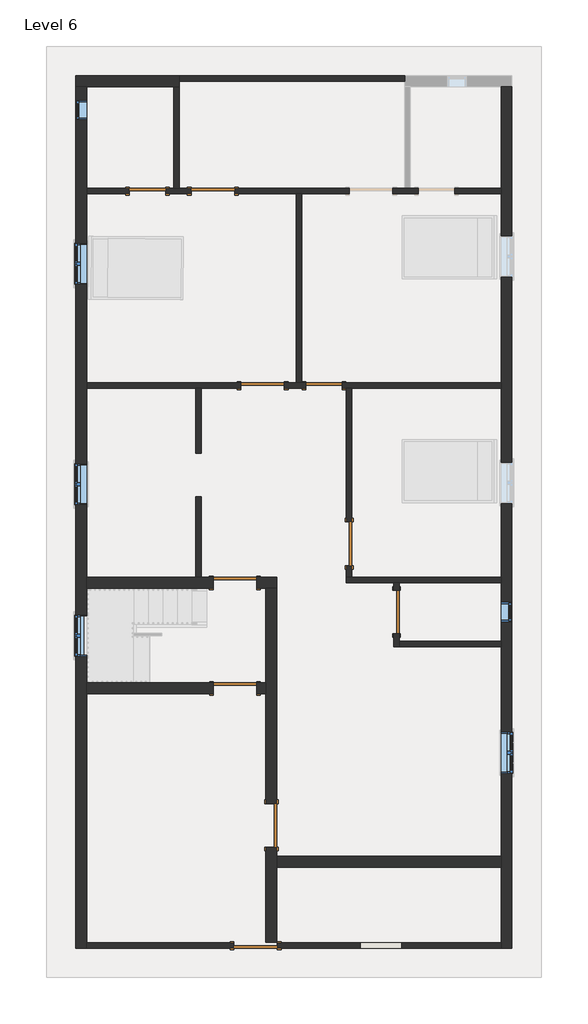
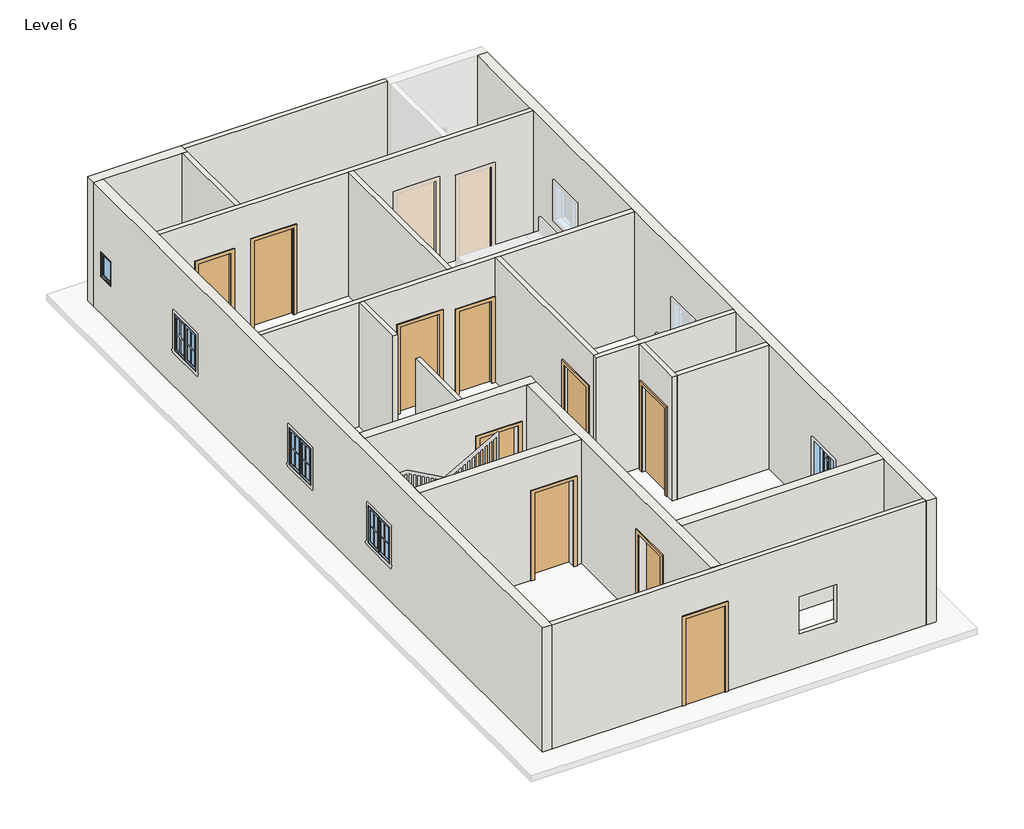
# One storey, part 1 of 3: 19 walls, 10 doors, 6 windows.
"""IFC4 building model written with IfcOpenShell, lengths in millimetres."""

from ifc_helpers import new_model, si_unit, frame, origin, place, context, project, spatial, polyline, outline, extrude, faceted_brep, transform, mapped, element, save
from components import door_d8f5dbb5, door_f2b275c1, door_e5f9f3c4, door_0ca8825f, door_305aa2a5, window_aa618e30, window_339605e1

model = new_model("IFC4")

# Units and contexts
model_context = context("Model", 3, world=origin())
ifc_project = project(units=[si_unit("LENGTHUNIT", "METRE", prefix="MILLI")], contexts=[model_context])

# Site, building, storey
site = spatial("IfcSite", under=ifc_project)
building = spatial("IfcBuilding", under=site)
storey = spatial("IfcBuildingStorey", under=building, Name="Level 6", Elevation=12801.6)

# Doors
placement = place(None, origin())
door_shape = door_d8f5dbb5(model_context)
element("IfcDoor", 1, ObjectType="Single-Flush : 30\" x 80\"", at=placement, inside=storey, context=model_context, shape_type="MappedRepresentation", body=[
    mapped(door_shape, transform((-4322.2915084, 8007.7072267, 12801.6), x_axis=(1.0, 0.0, 0.0), y_axis=(0.0, 1.0, 0.0), z_axis=(0.0, 0.0, 1.0))),
])
door_2_shape = door_f2b275c1(model_context)
element("IfcDoor", 2, ObjectType="Single-Flush : 30\" x 80\"", at=placement, inside=storey, context=model_context, shape_type="MappedRepresentation", body=[
    mapped(door_2_shape, transform((-621.124692, 3931.0072267, 12801.6), x_axis=(-1.0, 0.0, 0.0), y_axis=(0.0, -1.0, 0.0), z_axis=(0.0, 0.0, 1.0))),
])
door_3_shape = door_e5f9f3c4(model_context)
element("IfcDoor", 3, ObjectType="Single-Flush : 36\" x 84\"", at=placement, inside=storey, context=model_context, shape_type="MappedRepresentation", body=[
    mapped(door_3_shape, transform((-1909.2915084, 3931.0072267, 12801.6), x_axis=(1.0, 0.0, 0.0), y_axis=(0.0, 1.0, 0.0), z_axis=(0.0, 0.0, 1.0))),
])
element("IfcDoor", 4, ObjectType="Single-Flush : 36\" x 84\"", at=placement, inside=storey, context=model_context, shape_type="MappedRepresentation", body=[
    mapped(door_3_shape, transform((-94.9578757, 616.3072267, 12801.6), x_axis=(0.0, -1.0, 0.0), y_axis=(1.0, 0.0, 0.0), z_axis=(0.0, 0.0, 1.0))),
])
element("IfcDoor", 5, ObjectType="Single-Flush : 36\" x 84\"", at=placement, inside=storey, context=model_context, shape_type="MappedRepresentation", body=[
    mapped(door_3_shape, transform((-2055.3415084, -7803.7927733, 12801.6), x_axis=(-1.0, 0.0, 0.0), y_axis=(0.0, -1.0, 0.0), z_axis=(0.0, 0.0, 1.0))),
])
door_4_shape = door_0ca8825f(model_context)
element("IfcDoor", 6, ObjectType="Single-Flush : 36\" x 84\"", at=placement, inside=storey, context=model_context, shape_type="MappedRepresentation", body=[
    mapped(door_4_shape, transform((-2490.3165084, -202.8427733, 12801.6), x_axis=(1.0, 0.0, 0.0), y_axis=(0.0, 1.0, 0.0), z_axis=(0.0, 0.0, 1.0))),
])
element("IfcDoor", 7, ObjectType="Single-Flush : 36\" x 84\"", at=placement, inside=storey, context=model_context, shape_type="MappedRepresentation", body=[
    mapped(door_4_shape, transform((-2487.1415084, -2412.6427733, 12801.6), x_axis=(1.0, 0.0, 0.0), y_axis=(0.0, 1.0, 0.0), z_axis=(0.0, 0.0, 1.0))),
])
element("IfcDoor", 8, ObjectType="Single-Flush : 36\" x 84\"", at=placement, inside=storey, context=model_context, shape_type="MappedRepresentation", body=[
    mapped(door_4_shape, transform((-1725.1415084, -5282.8427733, 12801.6), x_axis=(0.0, -1.0, 0.0), y_axis=(1.0, 0.0, 0.0), z_axis=(0.0, 0.0, 1.0))),
])
door_5_shape = door_305aa2a5(model_context)
element("IfcDoor", 9, ObjectType="Single-Flush : 36\" x 84\"", at=placement, inside=storey, context=model_context, shape_type="MappedRepresentation", body=[
    mapped(door_5_shape, transform((897.4084916, -812.4427733, 12801.6), x_axis=(0.0, 1.0, 0.0), y_axis=(-1.0, 0.0, 0.0), z_axis=(0.0, 0.0, 1.0))),
])
element("IfcDoor", 10, ObjectType="Single-Flush : 36\" x 84\"", at=placement, inside=storey, context=model_context, shape_type="MappedRepresentation", body=[
    mapped(door_5_shape, transform((-2950.6915084, 8007.7072267, 12801.6), x_axis=(-1.0, 0.0, 0.0), y_axis=(0.0, -1.0, 0.0), z_axis=(0.0, 0.0, 1.0))),
])

# Walls
element("IfcWall", 11, ObjectType="WALL4.5\"", at=placement, inside=storey, context=model_context, shape_type="Brep", body=[
    faceted_brep([(821.2084916, 7950.5572267, 14935.2), (821.2084916, 7950.5572267, 12801.6), (1354.6084916, 7950.5572267, 12801.6), (1354.6084916, 7950.5572267, 14833.6), (2116.6084916, 7950.5572267, 14833.6), (2116.6084916, 7950.5572267, 12801.6), (3088.1584916, 7950.5572267, 12801.6), (3088.1584916, 7950.5572267, 15849.6), (-1090.1415084, 7950.5572267, 15849.6), (-1204.4415084, 7950.5572267, 15849.6), (-5598.6415084, 7950.5572267, 15849.6), (-5598.6415084, 7950.5572267, 12801.6), (-4703.2915084, 7950.5572267, 12801.6), (-4703.2915084, 7950.5572267, 14833.6), (-3941.2915084, 7950.5572267, 14833.6), (-3941.2915084, 7950.5572267, 12801.6), (-3407.8915084, 7950.5572267, 12801.6), (-3407.8915084, 7950.5572267, 14935.2), (-2493.4915084, 7950.5572267, 14935.2), (-2493.4915084, 7950.5572267, 12801.6), (-1204.4415084, 7950.5572267, 12801.6), (-1090.1415084, 7950.5572267, 12801.6), (-93.1915084, 7950.5572267, 12801.6), (-93.1915084, 7950.5572267, 14935.2), (1354.6084916, 8064.8572267, 12801.6), (1183.1584916, 8064.8572267, 12801.6), (1068.8584916, 8064.8572267, 12801.6), (821.2084916, 8064.8572267, 12801.6), (821.2084916, 8064.8572267, 14935.2), (-93.1915084, 8064.8572267, 14935.2), (-93.1915084, 8064.8572267, 12801.6), (-2493.4915084, 8064.8572267, 12801.6), (-2493.4915084, 8064.8572267, 14935.2), (-3407.8915084, 8064.8572267, 14935.2), (-3407.8915084, 8064.8572267, 12801.6), (-3655.5415084, 8064.8572267, 12801.6), (-3769.8415084, 8064.8572267, 12801.6), (-3941.2915084, 8064.8572267, 12801.6), (-3941.2915084, 8064.8572267, 14833.6), (-4703.2915084, 8064.8572267, 14833.6), (-4703.2915084, 8064.8572267, 12801.6), (-5598.6415084, 8064.8572267, 12801.6), (-5598.6415084, 8064.8572267, 15849.6), (-3769.8415084, 8064.8572267, 15849.6), (-3655.5415084, 8064.8572267, 15849.6), (1068.8584916, 8064.8572267, 15849.6), (1183.1584916, 8064.8572267, 15849.6), (3088.1584916, 8064.8572267, 15849.6), (3088.1584916, 8064.8572267, 12801.6), (2116.6084916, 8064.8572267, 12801.6), (2116.6084916, 8064.8572267, 14833.6), (1354.6084916, 8064.8572267, 14833.6)], [[[0, 1, 2, 3, 4, 5, 6, 7, 8, 9, 10, 11, 12, 13, 14, 15, 16, 17, 18, 19, 20, 21, 22, 23]], [[24, 25, 26, 27, 28, 29, 30, 31, 32, 33, 34, 35, 36, 37, 38, 39, 40, 41, 42, 43, 44, 45, 46, 47, 48, 49, 50, 51]], [[12, 11, 41, 40]], [[49, 48, 6, 5]], [[37, 36, 35, 34, 16, 15]], [[2, 1, 27, 26, 25, 24]], [[22, 21, 20, 19, 31, 30]], [[11, 10, 42, 41]], [[7, 6, 48, 47]], [[38, 37, 15, 14]], [[39, 38, 14, 13]], [[40, 39, 13, 12]], [[3, 2, 24, 51]], [[4, 3, 51, 50]], [[5, 4, 50, 49]], [[17, 16, 34, 33]], [[18, 17, 33, 32]], [[19, 18, 32, 31]], [[28, 27, 1, 0]], [[29, 28, 0, 23]], [[30, 29, 23, 22]], [[10, 9, 8, 7, 47, 46, 45, 44, 43, 42]]]),
])
element("IfcWall", 12, ObjectType="WALL4.5\"", at=placement, inside=storey, context=model_context, shape_type="SweptSolid", body=[
    extrude(outline(polyline([(-3769.8415084, 8064.8572267), (-3769.8415084, 10198.4572267), (-3655.5415084, 10198.4572267), (-3655.5415084, 8064.8572267), (-3769.8415084, 8064.8572267)])), frame((0.0, 0.0, 12801.6), z_axis=(0.0, 0.0, 1.0), x_axis=(1.0, 0.0, 0.0)), (0.0, 0.0, 1.0), 3048.0),
])
element("IfcWall", 13, ObjectType="WALL4.5\"", at=placement, inside=storey, context=model_context, shape_type="SweptSolid", body=[
    extrude(outline(polyline([(-1204.4415084, 3988.1572267), (-1204.4415084, 7950.5572267), (-1090.1415084, 7950.5572267), (-1090.1415084, 3988.1572267), (-1204.4415084, 3988.1572267)])), frame((0.0, 0.0, 12801.6), z_axis=(0.0, 0.0, 1.0), x_axis=(1.0, 0.0, 0.0)), (0.0, 0.0, 1.0), 3048.0),
])
element("IfcWall", 14, ObjectType="WALL4.5\"", at=placement, inside=storey, context=model_context, shape_type="Brep", body=[
    faceted_brep([(-1452.0915084, 3873.8572267, 12801.6), (-1002.124692, 3873.8572267, 12801.6), (-1002.124692, 3873.8572267, 14833.6), (-240.124692, 3873.8572267, 14833.6), (-240.124692, 3873.8572267, 12801.6), (-152.1078757, 3873.8572267, 12801.6), (-37.8078757, 3873.8572267, 12801.6), (3088.1584916, 3873.8572267, 12801.6), (3088.1584916, 3873.8572267, 15849.6), (-37.8078757, 3873.8572267, 15849.6), (-152.1078757, 3873.8572267, 15849.6), (-3198.3415084, 3873.8572267, 15849.6), (-3312.6415084, 3873.8572267, 15849.6), (-5598.6415084, 3873.8572267, 15849.6), (-5598.6415084, 3873.8572267, 12801.6), (-3312.6415084, 3873.8572267, 12801.6), (-3198.3415084, 3873.8572267, 12801.6), (-2366.4915084, 3873.8572267, 12801.6), (-2366.4915084, 3873.8572267, 14935.2), (-1452.0915084, 3873.8572267, 14935.2), (-1002.124692, 3988.1572267, 14833.6), (-1002.124692, 3988.1572267, 12801.6), (-1090.1415084, 3988.1572267, 12801.6), (-1204.4415084, 3988.1572267, 12801.6), (-1452.0915084, 3988.1572267, 12801.6), (-1452.0915084, 3988.1572267, 14935.2), (-2366.4915084, 3988.1572267, 14935.2), (-2366.4915084, 3988.1572267, 12801.6), (-5598.6415084, 3988.1572267, 12801.6), (-5598.6415084, 3988.1572267, 15849.6), (-1204.4415084, 3988.1572267, 15849.6), (-1090.1415084, 3988.1572267, 15849.6), (3088.1584916, 3988.1572267, 15849.6), (3088.1584916, 3988.1572267, 12801.6), (-240.124692, 3988.1572267, 12801.6), (-240.124692, 3988.1572267, 14833.6)], [[[0, 1, 2, 3, 4, 5, 6, 7, 8, 9, 10, 11, 12, 13, 14, 15, 16, 17, 18, 19]], [[20, 21, 22, 23, 24, 25, 26, 27, 28, 29, 30, 31, 32, 33, 34, 35]], [[17, 16, 15, 14, 28, 27]], [[34, 33, 7, 6, 5, 4]], [[24, 23, 22, 21, 1, 0]], [[14, 13, 29, 28]], [[8, 7, 33, 32]], [[25, 24, 0, 19]], [[26, 25, 19, 18]], [[27, 26, 18, 17]], [[2, 1, 21, 20]], [[3, 2, 20, 35]], [[4, 3, 35, 34]], [[13, 12, 11, 10, 9, 8, 32, 31, 30, 29]]]),
])
element("IfcWall", 15, ObjectType="WALL4.5\"", at=placement, inside=storey, context=model_context, shape_type="SweptSolid", body=[
    extrude(outline(polyline([(-3312.6415084, 2514.5843832), (-3312.6415084, 3873.8572267), (-3198.3415084, 3873.8572267), (-3198.3415084, 2514.5843832), (-3312.6415084, 2514.5843832)])), frame((0.0, 0.0, 12801.6), z_axis=(0.0, 0.0, 1.0), x_axis=(1.0, 0.0, 0.0)), (0.0, 0.0, 1.0), 3048.0),
])
element("IfcWall", 16, ObjectType="WALL4.5\"", at=placement, inside=storey, context=model_context, shape_type="SweptSolid", body=[
    extrude(outline(polyline([(-3312.6415084, -88.5427733), (-3312.6415084, 1600.2092553), (-3198.3415084, 1600.2092553), (-3198.3415084, -88.5427733), (-3312.6415084, -88.5427733)])), frame((0.0, 0.0, 12801.6), z_axis=(0.0, 0.0, 1.0), x_axis=(1.0, 0.0, 0.0)), (0.0, 0.0, 1.0), 3048.0),
])
element("IfcWall", 17, ObjectType="WALL4.5\"", at=placement, inside=storey, context=model_context, shape_type="SweptSolid", body=[
    extrude(outline(polyline([(159.1072267, 14935.2), (159.1072267, 12801.6), (-88.5427733, 12801.6), (-88.5427733, 15849.6), (3873.8572267, 15849.6), (3873.8572267, 12801.6), (1073.5072267, 12801.6), (1073.5072267, 14935.2), (159.1072267, 14935.2)])), frame((-152.1078757, 0.0, 0.0), z_axis=(1.0, 0.0, 0.0), x_axis=(0.0, 1.0, 0.0)), (0.0, 0.0, 1.0), 114.3),
])
element("IfcWall", 18, ObjectType="WALL4.5\"", at=placement, inside=storey, context=model_context, shape_type="Brep", body=[
    faceted_brep([(-152.1078757, -202.8427733, 12801.6), (840.2584916, -202.8427733, 12801.6), (954.5584916, -202.8427733, 12801.6), (3088.1584916, -202.8427733, 12801.6), (3088.1584916, -202.8427733, 15849.6), (954.5584916, -202.8427733, 15849.6), (840.2584916, -202.8427733, 15849.6), (-152.1078757, -202.8427733, 15849.6), (-152.1078757, -88.5427733, 12801.6), (-152.1078757, -88.5427733, 15849.6), (-37.8078757, -88.5427733, 15849.6), (3088.1584916, -88.5427733, 15849.6), (3088.1584916, -88.5427733, 12801.6), (-37.8078757, -88.5427733, 12801.6)], [[[0, 1, 2, 3, 4, 5, 6, 7]], [[8, 9, 10, 11, 12, 13]], [[3, 2, 1, 0, 8, 13, 12]], [[4, 3, 12, 11]], [[0, 7, 9, 8]], [[7, 6, 5, 4, 11, 10, 9]]]),
])
element("IfcWall", 19, ObjectType="WALL4.5\"", at=placement, inside=storey, context=model_context, shape_type="Brep", body=[
    faceted_brep([(840.2584916, -202.8427733, 12801.6), (840.2584916, -355.2427733, 12801.6), (840.2584916, -355.2427733, 14935.2), (840.2584916, -1269.6427733, 14935.2), (840.2584916, -1269.6427733, 12801.6), (840.2584916, -1536.3427733, 12801.6), (840.2584916, -1536.3427733, 15849.6), (840.2584916, -202.8427733, 15849.6), (954.5584916, -355.2427733, 14935.2), (954.5584916, -355.2427733, 12801.6), (954.5584916, -202.8427733, 12801.6), (954.5584916, -202.8427733, 15849.6), (954.5584916, -1422.0427733, 15849.6), (954.5584916, -1536.3427733, 15849.6), (954.5584916, -1536.3427733, 12801.6), (954.5584916, -1422.0427733, 12801.6), (954.5584916, -1269.6427733, 12801.6), (954.5584916, -1269.6427733, 14935.2)], [[[0, 1, 2, 3, 4, 5, 6, 7]], [[8, 9, 10, 11, 12, 13, 14, 15, 16, 17]], [[10, 9, 1, 0]], [[16, 15, 14, 5, 4]], [[0, 7, 11, 10]], [[6, 5, 14, 13]], [[2, 1, 9, 8]], [[3, 2, 8, 17]], [[4, 3, 17, 16]], [[7, 6, 13, 12, 11]]]),
])
element("IfcWall", 20, ObjectType="WALL4.5\"", at=placement, inside=storey, context=model_context, shape_type="SweptSolid", body=[
    extrude(outline(polyline([(3088.1584916, -1536.3427733), (954.5584916, -1536.3427733), (954.5584916, -1422.0427733), (3088.1584916, -1422.0427733), (3088.1584916, -1536.3427733)])), frame((0.0, 0.0, 12801.6), z_axis=(0.0, 0.0, 1.0), x_axis=(1.0, 0.0, 0.0)), (0.0, 0.0, 1.0), 3048.0),
])
element("IfcWall", 21, ObjectType="WALL4.5\"", at=placement, inside=storey, context=model_context, shape_type="SweptSolid", body=[
    extrude(outline(polyline([(12801.6, -5598.6415084), (12801.6, -2512.5415084), (14935.2, -2512.5415084), (14935.2, -1598.1415084), (12801.6, -1598.1415084), (12801.6, 3088.1584916), (15849.6, 3088.1584916), (15849.6, -5598.6415084), (12801.6, -5598.6415084)]), holes=[polyline([(14526.3479476, 141.7584916), (14526.3479476, 1005.3584916), (13611.9479476, 1005.3584916), (13611.9479476, 141.7584916), (14526.3479476, 141.7584916)])]), frame((0.0, -7860.9427733, 0.0), z_axis=(0.0, 1.0, 0.0), x_axis=(0.0, 0.0, 1.0)), (0.0, 0.0, 1.0), 114.3),
])
element("IfcWall", 22, ObjectType="WALL4.5\"", at=placement, inside=storey, context=model_context, shape_type="SweptSolid", body=[
    extrude(outline(polyline([(1068.8584916, 10312.7572267), (-3655.5415084, 10312.7572267), (-3655.5415084, 10427.0572267), (1068.8584916, 10427.0572267), (1068.8584916, 10312.7572267)])), frame((0.0, 0.0, 12801.6), z_axis=(0.0, 0.0, 1.0), x_axis=(1.0, 0.0, 0.0)), (0.0, 0.0, 1.0), 3048.0),
])
element("IfcWall", 23, ObjectType="WALL9\"", at=placement, inside=storey, context=model_context, shape_type="Brep", body=[
    faceted_brep([(-3655.5415084, 10427.0572267, 12801.6), (-5827.2415084, 10427.0572267, 12801.6), (-5827.2415084, 10427.0572267, 15849.6), (-3655.5415084, 10427.0572267, 15849.6), (-3655.5415084, 10198.4572267, 12801.6), (-3655.5415084, 10198.4572267, 15849.6), (-3769.8415084, 10198.4572267, 15849.6), (-5598.6415084, 10198.4572267, 15849.6), (-5827.2415084, 10198.4572267, 15849.6), (-5827.2415084, 10198.4572267, 12801.6), (-5598.6415084, 10198.4572267, 12801.6), (-3769.8415084, 10198.4572267, 12801.6), (-3655.5415084, 10312.7572267, 12801.6), (-3655.5415084, 10312.7572267, 15849.6)], [[[0, 1, 2, 3]], [[4, 5, 6, 7, 8, 9, 10, 11]], [[1, 0, 12, 4, 11, 10, 9]], [[2, 1, 9, 8]], [[0, 3, 13, 5, 4, 12]], [[3, 2, 8, 7, 6, 5, 13]]]),
])
element("IfcWall", 24, ObjectType="WALL9\"", at=placement, inside=storey, context=model_context, shape_type="Brep", body=[
    faceted_brep([(-5827.2415084, 10198.4572267, 12801.6), (-5827.2415084, -7860.9427733, 12801.6), (-5827.2415084, -7860.9427733, 15849.6), (-5827.2415084, 10198.4572267, 15849.6), (-5827.2415084, 9906.3572267, 14325.6), (-5827.2415084, 9499.9572267, 14325.6), (-5827.2415084, 9499.9572267, 13716.0), (-5827.2415084, 9906.3572267, 13716.0), (-5827.2415084, 6915.5072267, 14630.4), (-5827.2415084, 6051.9072267, 14630.4), (-5827.2415084, 6051.9072267, 13716.0), (-5827.2415084, 6915.5072267, 13716.0), (-5827.2415084, 2295.8822267, 14630.4), (-5827.2415084, 1432.2822267, 14630.4), (-5827.2415084, 1432.2822267, 13716.0), (-5827.2415084, 2295.8822267, 13716.0), (-5827.2415084, -875.9427733, 14630.4), (-5827.2415084, -1739.5427733, 14630.4), (-5827.2415084, -1739.5427733, 13716.0), (-5827.2415084, -875.9427733, 13716.0), (-5598.6415084, 10198.4572267, 12801.6), (-5598.6415084, 10198.4572267, 15849.6), (-5598.6415084, 8064.8572267, 15849.6), (-5598.6415084, 7950.5572267, 15849.6), (-5598.6415084, 3988.1572267, 15849.6), (-5598.6415084, 3873.8572267, 15849.6), (-5598.6415084, -88.5427733, 15849.6), (-5598.6415084, -317.1427733, 15849.6), (-5598.6415084, -2298.3427733, 15849.6), (-5598.6415084, -2526.9427733, 15849.6), (-5598.6415084, -7746.6427733, 15849.6), (-5598.6415084, -7860.9427733, 15849.6), (-5598.6415084, -7860.9427733, 12801.6), (-5598.6415084, -7746.6427733, 12801.6), (-5598.6415084, -2526.9427733, 12801.6), (-5598.6415084, -2298.3427733, 12801.6), (-5598.6415084, -317.1427733, 12801.6), (-5598.6415084, -88.5427733, 12801.6), (-5598.6415084, 3873.8572267, 12801.6), (-5598.6415084, 3988.1572267, 12801.6), (-5598.6415084, 7950.5572267, 12801.6), (-5598.6415084, 8064.8572267, 12801.6), (-5598.6415084, 9906.3572267, 14325.6), (-5598.6415084, 9906.3572267, 13716.0), (-5598.6415084, 9499.9572267, 13716.0), (-5598.6415084, 9499.9572267, 14325.6), (-5598.6415084, 6915.5072267, 14630.4), (-5598.6415084, 6915.5072267, 13716.0), (-5598.6415084, 6051.9072267, 13716.0), (-5598.6415084, 6051.9072267, 14630.4), (-5598.6415084, 2295.8822267, 14630.4), (-5598.6415084, 2295.8822267, 13716.0), (-5598.6415084, 1432.2822267, 13716.0), (-5598.6415084, 1432.2822267, 14630.4), (-5598.6415084, -875.9427733, 14630.4), (-5598.6415084, -875.9427733, 13716.0), (-5598.6415084, -1739.5427733, 13716.0), (-5598.6415084, -1739.5427733, 14630.4)], [[[0, 1, 2, 3], [4, 5, 6, 7], [8, 9, 10, 11], [12, 13, 14, 15], [16, 17, 18, 19]], [[20, 21, 22, 23, 24, 25, 26, 27, 28, 29, 30, 31, 32, 33, 34, 35, 36, 37, 38, 39, 40, 41], [42, 43, 44, 45], [46, 47, 48, 49], [50, 51, 52, 53], [54, 55, 56, 57]], [[1, 0, 20, 41, 40, 39, 38, 37, 36, 35, 34, 33, 32]], [[0, 3, 21, 20]], [[2, 1, 32, 31]], [[43, 42, 4, 7]], [[44, 43, 7, 6]], [[45, 44, 6, 5]], [[42, 45, 5, 4]], [[47, 46, 8, 11]], [[48, 47, 11, 10]], [[49, 48, 10, 9]], [[46, 49, 9, 8]], [[51, 50, 12, 15]], [[52, 51, 15, 14]], [[53, 52, 14, 13]], [[50, 53, 13, 12]], [[55, 54, 16, 19]], [[56, 55, 19, 18]], [[57, 56, 18, 17]], [[54, 57, 17, 16]], [[3, 2, 31, 30, 29, 28, 27, 26, 25, 24, 23, 22, 21]]]),
])
element("IfcWall", 25, ObjectType="WALL9\"", at=placement, inside=storey, context=model_context, shape_type="Brep", body=[
    faceted_brep([(3088.1584916, 10198.4572267, 12801.6), (3088.1584916, 8064.8572267, 12801.6), (3088.1584916, 7950.5572267, 12801.6), (3088.1584916, 3988.1572267, 12801.6), (3088.1584916, 3873.8572267, 12801.6), (3088.1584916, -88.5427733, 12801.6), (3088.1584916, -202.8427733, 12801.6), (3088.1584916, -1422.0427733, 12801.6), (3088.1584916, -1536.3427733, 12801.6), (3088.1584916, -5930.5427733, 12801.6), (3088.1584916, -6159.1427733, 12801.6), (3088.1584916, -7746.6427733, 12801.6), (3088.1584916, -7860.9427733, 12801.6), (3088.1584916, -7860.9427733, 15849.6), (3088.1584916, -7746.6427733, 15849.6), (3088.1584916, -6159.1427733, 15849.6), (3088.1584916, -5930.5427733, 15849.6), (3088.1584916, -1536.3427733, 15849.6), (3088.1584916, -1422.0427733, 15849.6), (3088.1584916, -202.8427733, 15849.6), (3088.1584916, -88.5427733, 15849.6), (3088.1584916, 3873.8572267, 15849.6), (3088.1584916, 3988.1572267, 15849.6), (3088.1584916, 7950.5572267, 15849.6), (3088.1584916, 8064.8572267, 15849.6), (3088.1584916, 10198.4572267, 15849.6), (3088.1584916, -1015.6427733, 14325.6), (3088.1584916, -1015.6427733, 13716.0), (3088.1584916, -609.2427733, 13716.0), (3088.1584916, -609.2427733, 14325.6), (3088.1584916, 6204.3072267, 14630.4), (3088.1584916, 6204.3072267, 13716.0), (3088.1584916, 7067.9072267, 13716.0), (3088.1584916, 7067.9072267, 14630.4), (3088.1584916, 1460.8572267, 14630.4), (3088.1584916, 1460.8572267, 13716.0), (3088.1584916, 2324.4572267, 13716.0), (3088.1584916, 2324.4572267, 14630.4), (3088.1584916, -4193.8177733, 14630.4), (3088.1584916, -4193.8177733, 13716.0), (3088.1584916, -3330.2177733, 13716.0), (3088.1584916, -3330.2177733, 14630.4), (3316.7584916, 10198.4572267, 12801.6), (3316.7584916, 10198.4572267, 15849.6), (3316.7584916, -7860.9427733, 15849.6), (3316.7584916, -7860.9427733, 12801.6), (3316.7584916, -1015.6427733, 14325.6), (3316.7584916, -609.2427733, 14325.6), (3316.7584916, -609.2427733, 13716.0), (3316.7584916, -1015.6427733, 13716.0), (3316.7584916, 6204.3072267, 14630.4), (3316.7584916, 7067.9072267, 14630.4), (3316.7584916, 7067.9072267, 13716.0), (3316.7584916, 6204.3072267, 13716.0), (3316.7584916, 1460.8572267, 14630.4), (3316.7584916, 2324.4572267, 14630.4), (3316.7584916, 2324.4572267, 13716.0), (3316.7584916, 1460.8572267, 13716.0), (3316.7584916, -4193.8177733, 14630.4), (3316.7584916, -3330.2177733, 14630.4), (3316.7584916, -3330.2177733, 13716.0), (3316.7584916, -4193.8177733, 13716.0)], [[[0, 1, 2, 3, 4, 5, 6, 7, 8, 9, 10, 11, 12, 13, 14, 15, 16, 17, 18, 19, 20, 21, 22, 23, 24, 25], [26, 27, 28, 29], [30, 31, 32, 33], [34, 35, 36, 37], [38, 39, 40, 41]], [[42, 43, 44, 45], [46, 47, 48, 49], [50, 51, 52, 53], [54, 55, 56, 57], [58, 59, 60, 61]], [[12, 11, 10, 9, 8, 7, 6, 5, 4, 3, 2, 1, 0, 42, 45]], [[0, 25, 43, 42]], [[13, 12, 45, 44]], [[27, 26, 46, 49]], [[28, 27, 49, 48]], [[29, 28, 48, 47]], [[26, 29, 47, 46]], [[31, 30, 50, 53]], [[32, 31, 53, 52]], [[33, 32, 52, 51]], [[30, 33, 51, 50]], [[35, 34, 54, 57]], [[36, 35, 57, 56]], [[37, 36, 56, 55]], [[34, 37, 55, 54]], [[39, 38, 58, 61]], [[40, 39, 61, 60]], [[41, 40, 60, 59]], [[38, 41, 59, 58]], [[25, 24, 23, 22, 21, 20, 19, 18, 17, 16, 15, 14, 13, 44, 43]]]),
])
element("IfcWall", 26, ObjectType="WALL9\"", at=placement, inside=storey, context=model_context, shape_type="Brep", body=[
    faceted_brep([(-2033.1165084, -317.1427733, 14935.2), (-2033.1165084, -317.1427733, 12801.6), (-1839.4415084, -317.1427733, 12801.6), (-1610.8415084, -317.1427733, 12801.6), (-1610.8415084, -317.1427733, 15849.6), (-1839.4415084, -317.1427733, 15849.6), (-5598.6415084, -317.1427733, 15849.6), (-5598.6415084, -317.1427733, 12801.6), (-2947.5165084, -317.1427733, 12801.6), (-2947.5165084, -317.1427733, 14935.2), (-1610.8415084, -88.5427733, 12801.6), (-2033.1165084, -88.5427733, 12801.6), (-2033.1165084, -88.5427733, 14935.2), (-2947.5165084, -88.5427733, 14935.2), (-2947.5165084, -88.5427733, 12801.6), (-3198.3415084, -88.5427733, 12801.6), (-3312.6415084, -88.5427733, 12801.6), (-5598.6415084, -88.5427733, 12801.6), (-5598.6415084, -88.5427733, 15849.6), (-3312.6415084, -88.5427733, 15849.6), (-3198.3415084, -88.5427733, 15849.6), (-1610.8415084, -88.5427733, 15849.6)], [[[0, 1, 2, 3, 4, 5, 6, 7, 8, 9]], [[10, 11, 12, 13, 14, 15, 16, 17, 18, 19, 20, 21]], [[8, 7, 17, 16, 15, 14]], [[3, 2, 1, 11, 10]], [[7, 6, 18, 17]], [[4, 3, 10, 21]], [[12, 11, 1, 0]], [[13, 12, 0, 9]], [[14, 13, 9, 8]], [[6, 5, 4, 21, 20, 19, 18]]]),
])
element("IfcWall", 27, ObjectType="WALL9\"", at=placement, inside=storey, context=model_context, shape_type="Brep", body=[
    faceted_brep([(-1839.4415084, -5740.0427733, 14935.2), (-1839.4415084, -5740.0427733, 12801.6), (-1839.4415084, -7733.9427733, 12801.6), (-1839.4415084, -7733.9427733, 15849.6), (-1839.4415084, -2526.9427733, 15849.6), (-1839.4415084, -2298.3427733, 15849.6), (-1839.4415084, -317.1427733, 15849.6), (-1839.4415084, -317.1427733, 12801.6), (-1839.4415084, -2298.3427733, 12801.6), (-1839.4415084, -2526.9427733, 12801.6), (-1839.4415084, -4825.6427733, 12801.6), (-1839.4415084, -4825.6427733, 14935.2), (-1610.8415084, -7733.9427733, 12801.6), (-1610.8415084, -6159.1427733, 12801.6), (-1610.8415084, -5930.5427733, 12801.6), (-1610.8415084, -5740.0427733, 12801.6), (-1610.8415084, -5740.0427733, 14935.2), (-1610.8415084, -4825.6427733, 14935.2), (-1610.8415084, -4825.6427733, 12801.6), (-1610.8415084, -317.1427733, 12801.6), (-1610.8415084, -317.1427733, 15849.6), (-1610.8415084, -5930.5427733, 15849.6), (-1610.8415084, -6159.1427733, 15849.6), (-1610.8415084, -7733.9427733, 15849.6)], [[[0, 1, 2, 3, 4, 5, 6, 7, 8, 9, 10, 11]], [[12, 13, 14, 15, 16, 17, 18, 19, 20, 21, 22, 23]], [[2, 1, 15, 14, 13, 12]], [[10, 9, 8, 7, 19, 18]], [[3, 2, 12, 23]], [[7, 6, 20, 19]], [[16, 15, 1, 0]], [[17, 16, 0, 11]], [[18, 17, 11, 10]], [[6, 5, 4, 3, 23, 22, 21, 20]]]),
])
element("IfcWall", 28, ObjectType="WALL9\"", at=placement, inside=storey, context=model_context, shape_type="SweptSolid", body=[
    extrude(outline(polyline([(3088.1584916, -6159.1427733), (-1610.8415084, -6159.1427733), (-1610.8415084, -5930.5427733), (3088.1584916, -5930.5427733), (3088.1584916, -6159.1427733)])), frame((0.0, 0.0, 12801.6), z_axis=(0.0, 0.0, 1.0), x_axis=(1.0, 0.0, 0.0)), (0.0, 0.0, 1.0), 3048.0),
])
element("IfcWall", 29, ObjectType="WALL9\"", at=placement, inside=storey, context=model_context, shape_type="SweptSolid", body=[
    extrude(outline(polyline([(14935.2, -2029.9415084), (12801.6, -2029.9415084), (12801.6, -1839.4415084), (15849.6, -1839.4415084), (15849.6, -5598.6415084), (12801.6, -5598.6415084), (12801.6, -2944.3415084), (14935.2, -2944.3415084), (14935.2, -2029.9415084)])), frame((0.0, -2526.9427733, 0.0), z_axis=(0.0, 1.0, 0.0), x_axis=(0.0, 0.0, 1.0)), (0.0, 0.0, 1.0), 228.6),
])

# Windows
window_shape = window_aa618e30(model_context)
element("IfcWindow", 30, ObjectType="Fixed : 16\" x 24\"", at=placement, inside=storey, context=model_context, shape_type="MappedRepresentation", body=[
    mapped(window_shape, transform((-5712.9415084, 9741.2572267, 12801.6), x_axis=(0.0, 1.0, 0.0), y_axis=(-1.0, 0.0, 0.0), z_axis=(0.0, 0.0, 1.0))),
])
element("IfcWindow", 31, ObjectType="Fixed : 16\" x 24\"", at=placement, inside=storey, context=model_context, shape_type="MappedRepresentation", body=[
    mapped(window_shape, transform((3202.4584916, -850.5427733, 12801.6), x_axis=(0.0, -1.0, 0.0), y_axis=(1.0, 0.0, 0.0), z_axis=(0.0, 0.0, 1.0))),
])
window_2_shape = window_339605e1(model_context)
element("IfcWindow", 32, ObjectType="Window-Casement-Double : 34\" x 36\"", at=placement, inside=storey, context=model_context, shape_type="MappedRepresentation", body=[
    mapped(window_2_shape, transform((-5712.9415084, 6483.7072267, 12801.6), x_axis=(0.0, 1.0, 0.0), y_axis=(-1.0, 0.0, 0.0), z_axis=(0.0, 0.0, 1.0))),
])
element("IfcWindow", 33, ObjectType="Window-Casement-Double : 34\" x 36\"", at=placement, inside=storey, context=model_context, shape_type="MappedRepresentation", body=[
    mapped(window_2_shape, transform((-5712.9415084, 1864.0822267, 12801.6), x_axis=(0.0, 1.0, 0.0), y_axis=(-1.0, 0.0, 0.0), z_axis=(0.0, 0.0, 1.0))),
])
element("IfcWindow", 34, ObjectType="Window-Casement-Double : 34\" x 36\"", at=placement, inside=storey, context=model_context, shape_type="MappedRepresentation", body=[
    mapped(window_2_shape, transform((3202.4584916, -3762.0177733, 12801.6), x_axis=(0.0, -1.0, 0.0), y_axis=(1.0, 0.0, 0.0), z_axis=(0.0, 0.0, 1.0))),
])
element("IfcWindow", 35, ObjectType="Window-Casement-Double : 34\" x 36\"", at=placement, inside=storey, context=model_context, shape_type="MappedRepresentation", body=[
    mapped(window_2_shape, transform((-5712.9415084, -1307.7427733, 12801.6), x_axis=(0.0, 1.0, 0.0), y_axis=(-1.0, 0.0, 0.0), z_axis=(0.0, 0.0, 1.0))),
])

save(model, "model.ifc")

# Revit data of these elements
# Type "Single-Flush : 30\" x 80\""
#   Type Mark = "5"
#   Construction Type Id = "MDOOR"
#   Assembly Code = "C1020"
#   Analytic Construction = "Metal"
#   Thickness = 0' - 2"
#   Heat Transfer Coefficient (U) = 0.651978 BTU/(h·ft²·°F)
#   Height = 6' - 8"
#   Trim Projection Ext = 0' - 1"
#   Trim Projection Int = 0' - 1"
#   Trim Width = 0' - 3"
#   Width = 2' - 6"
#   Define Thermal Properties by = 1
#   Define Thermal Properties by = 1
#   Door Material = Door - Panel
#   Frame Material = Door - Frame
#   Visual Light Transmittance = 0
#   Solar Heat Gain Coefficient = 0
#   Function = (empty or 0)
#   Wall Closure = (empty or 0)
# Type "Single-Flush : 36\" x 84\""
#   Type Mark = "1"
#   Construction Type Id = "MDOOR"
#   Assembly Code = "C1020"
#   Analytic Construction = "Metal"
#   Thickness = 0' - 2"
#   Heat Transfer Coefficient (U) = 0.651978 BTU/(h·ft²·°F)
#   Height = 7' - 0"
#   Trim Projection Ext = 0' - 1"
#   Trim Projection Int = 0' - 1"
#   Trim Width = 0' - 3"
#   Width = 3' - 0"
#   Define Thermal Properties by = 1
#   Define Thermal Properties by = 1
#   Door Material = Door - Panel
#   Frame Material = Door - Frame
#   Visual Light Transmittance = 0
#   Solar Heat Gain Coefficient = 0
#   Function = (empty or 0)
#   Wall Closure = (empty or 0)
# Type "WALL4.5\""
#   Assembly Code = "B2010"
#   Layers, outside or top first: 0' - 4 1/2" no material (function 1)
# Type "WALL9\""
#   Assembly Code = "B2010"
#   Layers, outside or top first: 0' - 9" no material (function 1)
# Type "Fixed : 16\" x 24\""
#   Type Mark = "4"
#   Construction Type Id = "GSP4R"
#   Assembly Code = "B2020100"
#   Analytic Construction = "1/8 in Pilkington single glazing"
#   Visual Light Transmittance = 0.9
#   Solar Heat Gain Coefficient = 0.78
#   Heat Transfer Coefficient (U) = 0.6496 BTU/(h·ft²·°F)
#   Height = 2' - 0"
#   Default Sill Height = 3' - 0"
#   Width = 1' - 4"
#   Window Inset = 0' - 0 3/4"
#   Define Thermal Properties by = 1
#   Define Thermal Properties by = 1
#   Glass Pane Material = Glass
#   Sash Material = Sash
#   Wall Closure = (empty or 0)
# Type "Window-Casement-Double : 34\" x 36\""
#   Type Mark = "14"
#   Fire Rating = "0.5h"
#   Assembly Code = "B2020100"
#   Analytic Construction = "Double glazing - domestic"
#   Frame Extension [instance default] = 0' - 0 1/4"
#   Window Inset [instance default] = 0' - 0"
#   Wall Thickness [instance default] = 0' - 6"
#   Interior Wall Closure [instance default] = 0' - 2 1/4"
#   Half Width = 1' - 5"
#   Visual Light Transmittance = 0.81
#   Thermal Resistance (R) = 1.8146 (h·ft²·°F)/BTU
#   Solar Heat Gain Coefficient = 0.76
#   Rough Width = 2' - 10 1/2"
#   Rough Height = 3' - 0 1/2"
#   Height = 3' - 0"
#   Heat Transfer Coefficient (U) = 0.5511 BTU/(h·ft²·°F)
#   Exterior Wall Closure [instance default] = 0' - 1 1/4"
#   Extension Jamb [instance default] = 0' - 2 1/4"
#   Default Sill Height = 3' - 0"
#   Width = 2' - 10"
#   Define Thermal Properties by = 0
#   Muntin Visibility = yes
#   Interior Trim Visibility [instance default] = yes
#   Exterior Trim Visibility [instance default] = yes
#   Extension Jamb Visibility [instance default] = yes
#   Interior Trim Material = Wood - Stained
#   Muntin Pattern = Muntin Pattern_2x2 : Muntin Pattern_2x2
#   Interior Trim = Trim-Window-Interior-Flat : Picture Frame
#   Interior Frame Material = Wood - Stained
#   Glass Panel Material = Glass
#   Exterior Trim Material = Clad - White
#   Exterior Trim = Trim-Window-Exterior-Flat : with Sill
#   Exterior Frame Material = Clad - White
#   Wall Closure = (empty or 0)
# Elements 1, 2 (IfcDoor, "Single-Flush : 30\" x 80\"")
#   Phase Created = New Construction
#   Materials on its faces: "Door - Frame", "Door - Panel"
# Elements 3, 4, 5, 6, 7, 8, 9, 10 (IfcDoor, "Single-Flush : 36\" x 84\"")
#   Phase Created = New Construction
#   Materials on its faces: "Door - Frame", "Door - Panel"
# Elements 11, 21, 22 (IfcWall, "WALL4.5\"")
#   Top Offset = 0' - 0"
#   Base Offset = 0' - 0"
#   Unconnected Height = 10' - 0"
#   wall height = 10' - 0"
#   Phase Created = New Construction
#   Base Constraint = Level 6
#   Materials on its faces: "Default Wall", "Wood Planks"
# Elements 12, 13, 14, 15, 16, 17, 18, 19, 20 (IfcWall, "WALL4.5\"")
#   Top Offset = 0' - 0"
#   Base Offset = 0' - 0"
#   Unconnected Height = 10' - 0"
#   wall height = 10' - 0"
#   Phase Created = New Construction
#   Base Constraint = Level 6
#   Materials on its faces: "Default Wall"
# Elements 23, 24, 25 (IfcWall, "WALL9\"")
#   Top Offset = 0' - 0"
#   Base Offset = 0' - 0"
#   Unconnected Height = 10' - 0"
#   wall height = 10' - 0"
#   Phase Created = New Construction
#   Base Constraint = Level 6
#   Materials on its faces: "Default Wall", "Wood Planks"
# Elements 26, 27, 28, 29 (IfcWall, "WALL9\"")
#   Top Offset = 0' - 0"
#   Base Offset = 0' - 0"
#   Unconnected Height = 10' - 0"
#   wall height = 10' - 0"
#   Phase Created = New Construction
#   Base Constraint = Level 6
#   Materials on its faces: "Default Wall"
# Element 30 (IfcWindow, "Fixed : 16\" x 24\"")
#   Mark = "37"
#   Phase Created = New Construction
#   Materials on its faces: "Sash", "Glass"
# Element 31 (IfcWindow, "Fixed : 16\" x 24\"")
#   Mark = "39"
#   Phase Created = New Construction
#   Materials on its faces: "Sash", "Glass"
# Element 32 (IfcWindow, "Window-Casement-Double : 34\" x 36\"")
#   Mark = "42"
#   Window Inset = 0' - 0"
#   Interior Wall Closure = 0' - 2 1/4"
#   Frame Extension = 0' - 0 1/4"
#   Exterior Wall Closure = 0' - 1 1/4"
#   Interior Trim Visibility = yes
#   Exterior Trim Visibility = yes
#   Phase Created = New Construction
#   Materials on its faces: "Wood - Stained", "Glass", "Clad - White"
# Element 33 (IfcWindow, "Window-Casement-Double : 34\" x 36\"")
#   Mark = "43"
#   Window Inset = 0' - 0"
#   Interior Wall Closure = 0' - 2 1/4"
#   Frame Extension = 0' - 0 1/4"
#   Exterior Wall Closure = 0' - 1 1/4"
#   Interior Trim Visibility = yes
#   Exterior Trim Visibility = yes
#   Phase Created = New Construction
#   Materials on its faces: "Wood - Stained", "Glass", "Clad - White"
# Element 34 (IfcWindow, "Window-Casement-Double : 34\" x 36\"")
#   Mark = "44"
#   Window Inset = 0' - 0"
#   Interior Wall Closure = 0' - 2 1/4"
#   Frame Extension = 0' - 0 1/4"
#   Exterior Wall Closure = 0' - 1 1/4"
#   Interior Trim Visibility = yes
#   Exterior Trim Visibility = yes
#   Phase Created = New Construction
#   Materials on its faces: "Wood - Stained", "Glass", "Clad - White"
# Element 35 (IfcWindow, "Window-Casement-Double : 34\" x 36\"")
#   Mark = "45"
#   Window Inset = 0' - 0"
#   Interior Wall Closure = 0' - 2 1/4"
#   Frame Extension = 0' - 0 1/4"
#   Exterior Wall Closure = 0' - 1 1/4"
#   Interior Trim Visibility = yes
#   Exterior Trim Visibility = yes
#   Phase Created = New Construction
#   Materials on its faces: "Wood - Stained", "Glass", "Clad - White"
# Materials
#   "Door - Panel": class "Wood", colour RGB 210 159 95, transparency 0, Cost = 0
#   "Door - Frame": colour RGB 118 70 51, transparency 0, Cost = 0
#   "Glass": class "Glass", colour RGB 0 128 192, transparency 0.75, Description = "Soda Lime Glass", Cost = 0
#   "Sash": class "Wood", colour RGB 224 178 126, transparency 0, Cost = 0
#   "Wood - Stained": class "Wood", colour RGB 224 178 126, transparency 0, Cost = 0
#   "Clad - White": class "Wood", colour RGB 242 242 238, transparency 0, Cost = 0
#   "Default Wall": colour RGB 128 128 128, transparency 0, Cost = 0
#   "Wood Planks": class "Wood", colour RGB 193 160 115, transparency 0, Description = "Physical material.", Cost = 0
